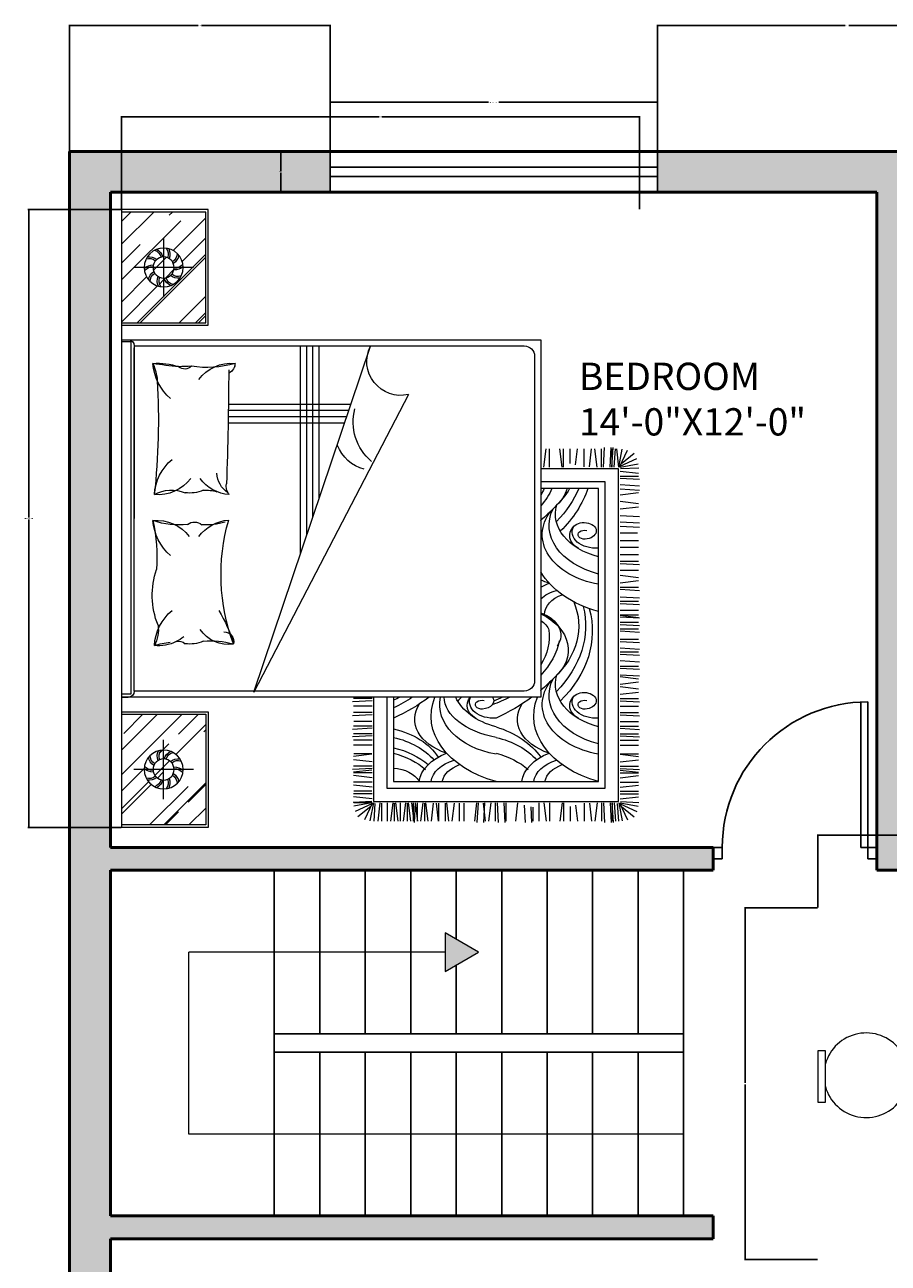
# Model space of a CAD drawing. Units: inches. Extents: x 2831 to 3729, y 3926 to 4974.
# Tile 3 of 8: x 2849 to 3038, y 4702 to 4974. Entities that reach past the tile are written whole.
import ezdxf

# ---------------------------------------------------------------- set-up
doc = ezdxf.new("R2010")
doc.units = ezdxf.units.IN
for name, color, linetype, lineweight in [('A-ANNO-DIMS', 2, 'Continuous', 18), ('A-ANNO-SYMB', 7, 'Continuous', 18), ('A-AREA-IDEN', 7, 'Continuous', 18), ('A-DOOR', 3, 'Continuous', 25), ('A-FLOR-STRS', 7, 'Continuous', 25), ('A-FURN', 8, 'Continuous', 18), ('A-GLAZ', 4, 'Continuous', 25), ('A-WALL', 7, 'Continuous', 50), ('A-WALL-PATT', 252, 'Continuous', 13)]:
    doc.layers.add(name, color=color, linetype=linetype, lineweight=lineweight)
doc.styles.get("Standard").update_dxf_attribs({"font": 'arial.ttf'})
doc.dimstyles.get("Standard").update_dxf_attribs({"dimtxt": 0.18, "dimasz": 0.18, "dimexe": 0.18, "dimexo": 0.0625, "dimgap": 0.09, "dimtad": 0, "dimtih": 1, "dimtoh": 1, "dimdec": 4, "dimzin": 0, "dimdsep": 46, "dimtxsty": 'Standard', "dimcen": 0.09, "dimadec": 0, "dimazin": 0, "dimtfac": 1, "dimtdec": 4, "dimtofl": 0, "dimtmove": 0, "dimatfit": 3, "dimfxl": 1, "dimtolj": 1, "dimtzin": 0, "dimarcsym": 0})

# ---------------------------------------------------------------- blocks, each defined once
blk = doc.blocks.new('A$C709B6AB6')
for p, q in [((0.969, 1.6731), (0.7259, 1.6731)), ((0.7259, 1.6731), (0.7259, 1.6374)), ((0.969, 1.6374), (0.969, 1.6731)), ((1.6452, 1.6731), (1.402, 1.6731)), ((1.402, 1.6731), (1.402, 1.6374)), ((1.6452, 1.6374), (1.6452, 1.6731)), ((0.7259, 1.6374), (0.969, 1.6374)), ((1.402, 1.6374), (1.6452, 1.6374)), ((0.3883, 0.3366), (0.3883, 1.3366)), ((0.3883, 1.3366), (1.9163, 1.3366)), ((0.4919, 1.2463), (0.4015, 1.3366)), ((0.7693, 1.0352), (0.468, 1.3366)), ((0.8475, 1.0774), (0.5883, 1.3366)), ((0.6526, 1.2956), (0.6117, 1.3366)), ((0.8205, 1.1564), (0.6404, 1.3366)), ((1.3746, 0.6706), (0.7087, 1.3366)), ((0.94, 1.1879), (0.7913, 1.3366)), ((1.0576, 1.108), (0.829, 1.3366)), ((1.4563, 0.7595), (0.9175, 1.2983)), ((1.1357, 1.1502), (0.9493, 1.3366)), ((1.2273, 1.0801), (0.9709, 1.3366)), ((1.6629, 0.7434), (1.0697, 1.3366)), ((1.486, 0.9688), (1.1182, 1.3366)), ((1.5147, 0.9724), (1.1505, 1.3366)), ((1.3459, 1.1807), (1.19, 1.3366)), ((1.424, 1.2229), (1.3103, 1.3366)), ((1.8021, 0.8646), (1.3531, 1.3136)), ((1.5156, 1.178), (1.357, 1.3366)), ((1.9163, 0.8509), (1.4307, 1.3366)), ((1.5506, 1.2956), (1.5097, 1.3366)), ((1.6341, 1.2534), (1.551, 1.3366)), ((1.8443, 1.0882), (1.5959, 1.3366)), ((1.7123, 1.2956), (1.6713, 1.3366)), ((1.838, 1.1879), (1.6893, 1.3366)), ((1.9163, 1.2119), (1.7917, 1.3366)), ((1.8739, 1.2974), (1.8348, 1.3366)), ((1.9163, 1.2891), (1.8689, 1.3366)), ((1.9163, 1.3322), (1.912, 1.3366)), ((1.9163, 0.3366), (1.9163, 1.3366)), ((1.0863, 0.5979), (0.3883, 1.296)), ((1.2525, 0.3366), (0.3883, 1.2008)), ((0.7909, 0.9472), (0.5215, 1.2166)), ((1.4321, 0.3366), (0.5448, 1.2238)), ((1.9163, 0.9299), (1.6404, 1.2058)), ((1.9163, 1.0916), (1.8021, 1.2058)), ((0.5592, 1.0047), (0.3883, 1.1756)), ((1.873, 0.7739), (1.5138, 1.1331)), ((1.8146, 0.879), (1.5452, 1.1484)), ((1.9163, 0.9712), (1.7599, 1.1277)), ((0.4622, 1.037), (0.3883, 1.111)), ((1.6117, 0.3366), (0.8322, 1.116)), ((1.4267, 0.5503), (0.8879, 1.0891)), ((0.4811, 0.9625), (0.3883, 1.0553)), ((1.0729, 0.3366), (0.3883, 1.0212)), ((0.7613, 0.738), (0.4919, 1.0074)), ((1.7913, 0.3366), (1.1196, 1.0083)), ((1.5847, 0.7012), (1.2255, 1.0604)), ((1.9163, 0.6102), (1.4716, 1.055)), ((1.9163, 1.0161), (1.9116, 1.0208)), ((0.0357, 0.9927), (0, 0.9927)), ((0, 0.9927), (0, 0.7495)), ((0.0357, 0.7495), (0.0357, 0.9927)), ((1.2965, 0.6284), (0.9373, 0.9876)), ((1.829, 0.3366), (1.1833, 0.9822)), ((2.269, 0.9927), (2.3047, 0.9927)), ((2.269, 0.7495), (2.269, 0.9927)), ((2.3047, 0.9927), (2.3047, 0.7495)), ((0.7981, 0.5251), (0.3883, 0.935)), ((1.0082, 0.5557), (0.649, 0.9149)), ((1.468, 0.3366), (0.8951, 0.9095)), ((1.9163, 0.3911), (1.4069, 0.9005)), ((1.785, 0.6697), (1.5156, 0.9391)), ((0.4326, 0.8278), (0.3883, 0.8721)), ((0.8933, 0.3366), (0.3883, 0.8416)), ((1.107, 0.3366), (0.6068, 0.8368)), ((1.3971, 0.341), (0.8582, 0.8799)), ((0.7199, 0.4829), (0.3883, 0.8146)), ((0.7316, 0.5287), (0.4622, 0.7981)), ((1.9163, 0.5707), (1.6943, 0.7927)), ((1.9163, 0.7773), (1.882, 0.8116)), ((0, 0.7495), (0.0357, 0.7495)), ((1.7554, 0.4605), (1.486, 0.7299)), ((2.3047, 0.7495), (2.269, 0.7495)), ((0.746, 0.3366), (0.3883, 0.6943)), ((0.7136, 0.3366), (0.3883, 0.662)), ((1.1627, 0.3366), (0.8286, 0.6706)), ((1.9163, 0.4899), (1.7527, 0.6536)), ((0.4029, 0.6185), (0.3883, 0.6332)), ((1.9163, 0.5384), (1.8524, 0.6024)), ((0.5098, 0.4524), (0.3883, 0.5739)), ((0.6849, 0.3366), (0.4326, 0.5889)), ((1.7087, 0.3366), (1.4644, 0.5808)), ((1.9163, 0.3696), (1.7105, 0.5754)), ((0.455, 0.4156), (0.3883, 0.4823)), ((1.3477, 0.3366), (1.1761, 0.5081)), ((1.5883, 0.3366), (1.4222, 0.5027)), ((1.6404, 0.3366), (1.4563, 0.5206)), ((0.4317, 0.4102), (0.3883, 0.4536)), ((0.9238, 0.3366), (0.799, 0.4614)), ((0.9866, 0.3366), (0.8879, 0.4353)), ((1.2273, 0.3366), (1.1339, 0.4299)), ((0.446, 0.3366), (0.4029, 0.3797)), ((0.6256, 0.3366), (0.5996, 0.3626)), ((0.8663, 0.3366), (0.8457, 0.3572)), ((1.8793, 0.3366), (1.8227, 0.3931)), ((1.9163, 0.3366), (0.3883, 0.3366)), ((0.7212, 0), (0.7212, 0.0357)), ((0.7212, 0.0357), (0.9644, 0.0357)), ((0.9644, 0.0357), (0.9644, 0)), ((1.3973, 0), (1.3973, 0.0357)), ((1.3973, 0.0357), (1.6405, 0.0357)), ((1.6405, 0.0357), (1.6405, 0)), ((0.9644, 0), (0.7212, 0)), ((1.6405, 0), (1.3973, 0))]:
    blk.add_line(p, q)
for centre, start, end in [((0.8475, 1.4434), 105.52104, 212.06337), ((0.8475, 1.4434), 327.93663, 74.47896), ((1.5236, 1.4434), 105.52104, 212.06337), ((1.5236, 1.4434), 327.93663, 74.47896), ((0.2296, 0.8768), 37.97614, 164.47896), ((2.075, 0.8768), 15.52104, 142.02386), ((0.2296, 0.8768), 195.52104, 322.02386), ((2.075, 0.8768), 217.97614, 344.47896), ((0.8428, 0.2297), 147.93663, 254.47896), ((0.8428, 0.2297), 285.52104, 32.06337), ((1.5189, 0.2297), 147.93663, 254.47896), ((1.5189, 0.2297), 285.52104, 32.06337)]:
    blk.add_arc(centre, 0.2013, start, end)
blk = doc.blocks.new('A$C64B41DC1')
for p, q in [((0, 2.5079), (2.9903, 2.5079)), ((0, 2.0879), (0, 2.5079)), ((0.012, 2.4618), (0.0581, 2.5079)), ((0.012, 2.3515), (0.1684, 2.5079)), ((0.012, 2.0999), (0.012, 2.5079)), ((0.0543, 2.2213), (0.3409, 2.5079)), ((0.1689, 2.4179), (0.2589, 2.5079)), ((0.3265, 2.386), (0.4484, 2.5079)), ((0.3699, 2.3332), (0.5445, 2.5079)), ((0.548, 2.5079), (0.548, 2.0999)), ((0.56, 2.5079), (0.56, 2.0879)), ((0.6301, 2.5079), (0.6301, 0.4779)), ((0.6401, 2.461), (0.6401, 2.5079)), ((0.6401, 2.5079), (2.344, 2.5079)), ((2.344, 2.461), (0.6401, 2.461)), ((2.344, 2.5079), (2.3601, 2.5079)), ((2.344, 2.5079), (2.344, 2.461)), ((2.3601, 2.5079), (2.3601, 2.4761)), ((2.3601, 0.4779), (2.3601, 2.5079)), ((2.4303, 2.5079), (2.4303, 2.0879)), ((2.4423, 2.5079), (2.4423, 2.0999)), ((2.4423, 2.3333), (2.6169, 2.5079)), ((2.4423, 2.2145), (2.7357, 2.5079)), ((2.4423, 2.404), (2.5354, 2.4971)), ((2.705, 2.398), (2.8149, 2.5079)), ((2.7691, 2.3772), (2.8998, 2.5079)), ((2.7819, 2.3646), (2.9252, 2.5079)), ((2.9783, 2.0999), (2.9783, 2.5079)), ((2.9903, 2.0879), (2.9903, 2.5079)), ((0.2157, 2.0999), (0.548, 2.4322)), ((0.2299, 2.0999), (0.548, 2.418)), ((0.2804, 2.1597), (0.2804, 2.4481)), ((0.6601, 2.4461), (1.4951, 2.4461)), ((0.6601, 2.4461), (0.6601, 0.5579)), ((1.4951, 2.4461), (0.6697, 2.4461)), ((2.3301, 2.4461), (1.4951, 2.4461)), ((2.3301, 0.5579), (2.3301, 2.4461)), ((2.7099, 2.1597), (2.7099, 2.4481)), ((0.2311, 2.2906), (0.2937, 2.3532)), ((2.6674, 2.2756), (2.7382, 2.3464)), ((2.7914, 2.1846), (2.9783, 2.3715)), ((0.1362, 2.3039), (0.4246, 2.3039)), ((0.2905, 2.2539), (0.3304, 2.2938)), ((0.3405, 2.3039), (0.3605, 2.3238)), ((2.8541, 2.3039), (2.5657, 2.3039)), ((2.5849, 2.2779), (2.6158, 2.3088)), ((2.6158, 2.3088), (2.6313, 2.3243)), ((2.7249, 2.3076), (2.7512, 2.3339)), ((2.7746, 2.0999), (2.9783, 2.3036)), ((2.9144, 2.2312), (2.9783, 2.2951)), ((0.012, 2.261), (0.0275, 2.2765)), ((0.0404, 2.0999), (0.1982, 2.2578)), ((0.4194, 2.0999), (0.548, 2.2285)), ((2.4423, 2.1353), (2.5382, 2.2312)), ((2.4918, 2.0999), (2.6366, 2.2447)), ((0.1365, 2.0999), (0.251, 2.2144)), ((2.7831, 2.0999), (2.8678, 2.1846)), ((2.8962, 2.0999), (2.9783, 2.182)), ((0.548, 2.0999), (0.012, 2.0999)), ((0.4986, 2.0999), (0.548, 2.1493)), ((0.5127, 2.0999), (0.548, 2.1352)), ((2.4423, 2.0999), (2.9783, 2.0999)), ((2.5172, 2.0999), (2.5269, 2.1096)), ((0.56, 2.0879), (0, 2.0879)), ((2.4303, 2.0879), (2.9903, 2.0879)), ((0.9415, 1.9902), (0.9415, 1.3975)), ((0.9715, 1.9906), (0.9715, 1.4076)), ((1.0015, 1.991), (1.0015, 1.4177)), ((1.0315, 1.9916), (1.0315, 1.4279)), ((2.3349, 1.8678), (0.6613, 1.3029)), ((0.8956, 1.1191), (2.3349, 1.8678)), ((1.6636, 1.6412), (0.6601, 1.6412)), ((1.5748, 1.6112), (0.6601, 1.6112)), ((2.3665, 1.295), (2.3665, 1.3839)), ((2.377, 1.295), (2.3822, 1.3891)), ((2.4032, 1.295), (2.4032, 1.3839)), ((2.4346, 1.295), (2.4346, 1.3839)), ((2.4451, 1.295), (2.4503, 1.3891)), ((2.4774, 1.2957), (2.4774, 1.3837)), ((2.5, 1.295), (2.5, 1.3839)), ((2.5105, 1.295), (2.5157, 1.3891)), ((2.5367, 1.295), (2.5367, 1.3839)), ((2.5471, 1.295), (2.5524, 1.3891)), ((2.5681, 1.295), (2.5681, 1.3839)), ((2.5918, 1.295), (2.5918, 1.3839)), ((2.6346, 1.2957), (2.6346, 1.3837)), ((2.6362, 1.2957), (2.6467, 1.3839)), ((2.6729, 1.295), (2.6624, 1.3839)), ((2.6938, 1.295), (2.6938, 1.3839)), ((2.7043, 1.295), (2.7095, 1.3891)), ((2.7127, 1.2957), (2.7232, 1.3839)), ((2.7253, 1.295), (2.7253, 1.3839)), ((2.7494, 1.295), (2.7389, 1.3839)), ((2.7718, 1.295), (2.7718, 1.3839)), ((2.7959, 1.295), (2.7854, 1.3839)), ((2.8146, 1.2957), (2.8146, 1.3837)), ((2.8146, 1.2957), (2.8146, 1.3837)), ((2.8282, 1.295), (2.8282, 1.3839)), ((2.8282, 1.295), (2.8282, 1.3839)), ((2.8523, 1.295), (2.8418, 1.3839)), ((2.8523, 1.295), (2.8418, 1.3839)), ((2.8653, 1.2966), (2.8688, 1.3861)), ((2.8711, 1.2957), (2.8711, 1.3837)), ((2.8711, 1.2957), (2.8875, 1.3822)), ((2.8713, 1.2927), (2.954, 1.3315)), ((2.8765, 1.2958), (2.9132, 1.3758)), ((2.8893, 1.3011), (2.9394, 1.3636)), ((2.3601, 1.2873), (2.8639, 1.2873)), ((2.8639, 1.2873), (2.8639, 0.1018)), ((2.8716, 1.2565), (2.9605, 1.2669)), ((2.8717, 1.2884), (2.9588, 1.3058)), ((2.8744, 1.2817), (2.9603, 1.2869)), ((2.3601, 1.2233), (2.7999, 1.2233)), ((2.7999, 1.2233), (2.7999, 0.1658)), ((2.8716, 1.2212), (2.9605, 1.2212)), ((2.8716, 1.1947), (2.9605, 1.2052)), ((2.8723, 1.2489), (2.9603, 1.2489)), ((2.3601, 1.1913), (2.7679, 1.1912)), ((2.7679, 1.1912), (2.7679, 0.1978)), ((2.8716, 1.181), (2.9605, 1.1705)), ((2.8716, 1.1595), (2.9605, 1.1595)), ((2.8716, 1.133), (2.9605, 1.1435)), ((2.8723, 1.1872), (2.9603, 1.1872)), ((2.8716, 1.1193), (2.9605, 1.1088)), ((2.8716, 1.1035), (2.9605, 1.093)), ((2.8716, 1.0965), (2.9605, 1.0965)), ((2.8716, 1.086), (2.9657, 1.0913)), ((2.8723, 1.1255), (2.9603, 1.1255)), ((2.8723, 1.0858), (2.9605, 1.0753)), ((2.8716, 1.0756), (2.9605, 1.0756)), ((2.8716, 1.0491), (2.9605, 1.0596)), ((2.8716, 1.0354), (2.9605, 1.0249)), ((2.8723, 1.0416), (2.9603, 1.0416)), ((2.8723, 0.9987), (2.9605, 1.0092)), ((2.8723, 0.985), (2.9605, 0.9745)), ((2.8723, 0.9735), (2.9603, 0.9735)), ((2.8716, 0.9346), (2.9605, 0.9241)), ((2.8723, 0.9408), (2.9603, 0.9408)), ((2.8723, 0.8979), (2.9605, 0.9084)), ((2.8723, 0.8726), (2.9603, 0.8726)), ((2.8723, 0.8505), (2.9603, 0.8505)), ((2.8716, 0.7885), (2.9605, 0.799)), ((2.8716, 0.7818), (2.9657, 0.787)), ((2.8716, 0.7503), (2.9657, 0.7556)), ((2.8716, 0.7204), (2.9605, 0.7309)), ((2.8723, 0.7571), (2.9605, 0.7466)), ((2.8716, 0.6995), (2.9605, 0.6995)), ((2.8716, 0.689), (2.9657, 0.6838)), ((2.8716, 0.6576), (2.9657, 0.6523)), ((2.8716, 0.6471), (2.9605, 0.6471)), ((2.8716, 0.5903), (2.9605, 0.6007)), ((2.882, 0.5582), (2.9657, 0.5536)), ((0.7101, 0.5079), (2.2801, 0.5079)), ((2.8716, 0.4877), (2.9603, 0.4877)), ((2.8909, 0.5263), (2.9657, 0.5222)), ((2.8928, 0.5169), (2.9605, 0.5169)), ((0.6301, 0.4779), (2.3601, 0.4779)), ((1.2465, 0.4625), (1.1576, 0.452)), ((1.2465, 0.4365), (1.1577, 0.4365)), ((1.2542, 0.1018), (1.2542, 0.4779)), ((1.3182, 0.1658), (1.3182, 0.4779)), ((1.3502, 0.1978), (1.3502, 0.4779)), ((2.8716, 0.4625), (2.9605, 0.452)), ((2.8716, 0.4365), (2.9603, 0.4365)), ((1.2465, 0.3746), (1.1576, 0.3851)), ((1.2465, 0.3684), (1.1577, 0.3684)), ((2.8716, 0.3746), (2.9605, 0.3851)), ((2.8716, 0.3684), (2.9603, 0.3684)), ((1.2355, 0.3092), (1.1576, 0.3)), ((1.2285, 0.3357), (1.1577, 0.3357)), ((2.8826, 0.3092), (2.9605, 0.3)), ((2.8896, 0.3357), (2.9603, 0.3357)), ((1.2457, 0.2423), (1.1576, 0.2319)), ((1.2457, 0.2676), (1.1577, 0.2676)), ((2.8723, 0.2676), (2.9603, 0.2676)), ((2.8723, 0.2423), (2.9605, 0.2319)), ((1.2465, 0.2057), (1.1576, 0.2161)), ((1.2465, 0.1847), (1.1576, 0.1847)), ((2.7679, 0.1978), (1.3502, 0.1978)), ((2.8716, 0.2057), (2.9605, 0.2161)), ((2.8716, 0.1847), (2.9605, 0.1847)), ((1.2465, 0.1742), (1.1524, 0.169)), ((1.2465, 0.1428), (1.1524, 0.1376)), ((1.2465, 0.1334), (1.1524, 0.1281)), ((1.2465, 0.1323), (1.1576, 0.1323)), ((1.2465, 0.1323), (1.1576, 0.1323)), ((1.2465, 0.1229), (1.1588, 0.1168)), ((2.7999, 0.1658), (1.3182, 0.1658)), ((2.8716, 0.1742), (2.9657, 0.169)), ((2.8716, 0.1428), (2.9657, 0.1376)), ((2.8716, 0.1334), (2.9657, 0.1281)), ((2.8716, 0.1323), (2.9605, 0.1323)), ((2.8716, 0.1229), (2.9593, 0.1168)), ((1.2465, 0.1), (1.1576, 0.1105)), ((1.2464, 0.1007), (1.1592, 0.0833)), ((1.2468, 0.0964), (1.1641, 0.0576)), ((1.2288, 0.088), (1.1787, 0.0255)), ((1.2415, 0.0933), (1.2049, 0.0133)), ((1.247, 0.0934), (1.2306, 0.0069)), ((1.2527, 0.0925), (1.2493, 0.003)), ((2.8639, 0.1018), (1.2542, 0.1018)), ((1.2658, 0.0941), (1.2762, 0.0052)), ((1.2899, 0.0941), (1.2899, 0.0052)), ((1.2999, 0.0941), (1.3051, 0)), ((1.3313, 0.0941), (1.3365, 0)), ((1.3523, 0.0941), (1.3575, 0)), ((1.3804, 0.0941), (1.3699, 0.0052)), ((1.4119, 0.0934), (1.4223, 0.0052)), ((1.4485, 0.0941), (1.438, 0.0052)), ((1.48, 0.0941), (1.4852, 0)), ((1.5114, 0.0941), (1.5166, 0)), ((1.5323, 0.0941), (1.5376, 0)), ((1.5638, 0.0941), (1.5638, 0.0105)), ((1.6021, 0.0941), (1.6021, 0.0052)), ((1.6336, 0.0941), (1.6336, 0.0052)), ((1.6702, 0.0941), (1.6702, 0.0052)), ((1.7017, 0.0941), (1.7017, 0.0052)), ((1.7122, 0.0941), (1.7174, 0)), ((1.7445, 0.0934), (1.7445, 0.0054)), ((1.7698, 0.0934), (1.7803, 0.0052)), ((1.8065, 0.0941), (1.796, 0.0052)), ((1.8274, 0.0941), (1.8274, 0.0052)), ((1.8379, 0.0941), (1.8431, 0)), ((1.8746, 0.0941), (1.8798, 0)), ((1.8955, 0.0941), (1.8955, 0.0052)), ((1.906, 0.0941), (1.9113, 0)), ((1.9384, 0.0934), (1.9384, 0.0054)), ((1.9609, 0.0941), (1.9609, 0.0052)), ((1.9636, 0.0934), (1.9741, 0.0052)), ((1.9714, 0.0941), (1.9766, 0)), ((1.9976, 0.0941), (1.9976, 0.0052)), ((2.0081, 0.0941), (2.0133, 0)), ((2.029, 0.0941), (2.029, 0.0052)), ((2.0395, 0.0941), (2.0447, 0)), ((2.0797, 0.0941), (2.0797, 0.0052)), ((2.0902, 0.0941), (2.0954, 0)), ((2.1216, 0.0941), (2.1269, 0)), ((2.1412, 0.0941), (2.1412, 0.0052)), ((2.1517, 0.0941), (2.1569, 0)), ((2.1831, 0.0941), (2.1884, 0)), ((2.2093, 0.0941), (2.2093, 0.0052)), ((2.2198, 0.0941), (2.225, 0)), ((2.2512, 0.0941), (2.2565, 0)), ((2.2603, 0.0934), (2.2707, 0.0052)), ((2.2969, 0.0941), (2.2864, 0.0052)), ((2.3089, 0.0934), (2.3193, 0.0052)), ((2.3455, 0.0941), (2.3351, 0.0052)), ((2.3665, 0.0941), (2.3665, 0.0052)), ((2.377, 0.0941), (2.3822, 0)), ((2.4032, 0.0941), (2.4032, 0.0052)), ((2.4346, 0.0941), (2.4346, 0.0052)), ((2.4451, 0.0941), (2.4503, 0)), ((2.4774, 0.0934), (2.4774, 0.0054)), ((2.5, 0.0941), (2.5, 0.0052)), ((2.5105, 0.0941), (2.5157, 0)), ((2.5367, 0.0941), (2.5367, 0.0052)), ((2.5471, 0.0941), (2.5524, 0)), ((2.5681, 0.0941), (2.5681, 0.0052)), ((2.5918, 0.0941), (2.5918, 0.0052)), ((2.6346, 0.0934), (2.6346, 0.0054)), ((2.6362, 0.0934), (2.6467, 0.0052)), ((2.6729, 0.0941), (2.6624, 0.0052)), ((2.6938, 0.0941), (2.6938, 0.0052)), ((2.7043, 0.0941), (2.7095, 0)), ((2.7127, 0.0934), (2.7232, 0.0052)), ((2.7253, 0.0941), (2.7253, 0.0052)), ((2.7494, 0.0941), (2.7389, 0.0052)), ((2.7718, 0.0941), (2.7718, 0.0052)), ((2.7959, 0.0941), (2.7854, 0.0052)), ((2.8146, 0.0934), (2.8146, 0.0054)), ((2.8282, 0.0941), (2.8282, 0.0052)), ((2.8523, 0.0941), (2.8418, 0.0052)), ((2.8653, 0.0925), (2.8688, 0.003)), ((2.8711, 0.0934), (2.8875, 0.0069)), ((2.8713, 0.0964), (2.954, 0.0576)), ((2.8717, 0.1007), (2.9588, 0.0833)), ((2.8744, 0.1074), (2.9603, 0.1022)), ((2.8765, 0.0933), (2.9132, 0.0133)), ((2.8893, 0.088), (2.9394, 0.0255))]:
    blk.add_line(p, q)
at = {"ltscale": 10}
for p, q in [((1.4859, 1.5812), (0.6601, 1.5812)), ((1.397, 1.5512), (0.6601, 1.5512))]:
    blk.add_line(p, q, dxfattribs=at)
for centre, radius in [((0.2804, 2.3039), 0.0942), ((2.7099, 2.3039), 0.0942), ((0.2804, 2.3039), 0.051), ((2.7099, 2.3039), 0.051)]:
    blk.add_circle(centre, radius)
for centre, radius, start, end in [((0.6601, 2.4761), 0.03, 180, 270), ((2.3301, 2.4761), 0.03, 270, 0), ((0.3286, 2.3561), 0.0605, 136.17003, 182.48975), ((2.6617, 2.3561), 0.0605, 357.51025, 43.82997), ((0.2417, 2.3614), 0.0462, 196.30017, 256.53802), ((0.2887, 2.3745), 0.0605, 172.17003, 218.48975), ((0.2828, 2.3731), 0.0462, 160.30017, 220.53802), ((0.3231, 2.3585), 0.0462, 124.30017, 184.53802), ((0.3501, 2.3178), 0.0605, 100.17003, 146.48975), ((0.347, 2.323), 0.0462, 88.30017, 148.53802), ((1.0526, 2.3302), 0.3085, 175.30484, 198.69419), ((-0.8702, 2.0941), 1.6364, 4.80985, 9.18918), ((0.8579, 2.6278), 0.2948, 247.51785, 264.26696), ((0.728, 2.111), 0.245, 40.4189, 85.9871), ((1.0164, 5.7096), 3.3803, 266.81337, 276.16021), ((1.3963, 2.1044), 0.245, 94.0129, 139.5811), ((1.1858, 2.3288), 0.1943, 306.5711, 5.88998), ((1.5348, 2.2652), 0.1767, 151.77364, 201.69827), ((1.6986, 2.3355), 0.1943, 174.11002, 233.4289), ((1.1481, 2.2311), 0.3783, 353.49469, 19.18669), ((1.6871, 3.192), 0.8561, 257.74383, 273.62843), ((1.4882, 2.111), 0.245, 40.4189, 85.9871), ((1.8674, 1.9709), 0.3878, 68.20259, 108.9817), ((2.1269, 2.1044), 0.245, 94.0129, 139.5811), ((2.0342, 2.4856), 0.1563, 261.59582, 298.90918), ((1.9165, 2.3288), 0.1943, 333.73715, 5.88998), ((2.6058, 2.2028), 0.517, 163.60457, 172.3273), ((2.6433, 2.323), 0.0462, 31.46198, 91.69983), ((2.6402, 2.3178), 0.0605, 33.51025, 79.82997), ((2.6672, 2.3585), 0.0462, 355.46198, 55.69983), ((2.7075, 2.3731), 0.0462, 319.46198, 19.69983), ((2.7016, 2.3745), 0.0605, 321.51025, 7.82997), ((2.7486, 2.3614), 0.0462, 283.46198, 343.69983), ((0.2153, 2.3276), 0.0462, 232.30017, 292.53802), ((0.2158, 2.3336), 0.0605, 244.17003, 290.48975), ((0.2457, 2.3659), 0.0605, 208.17003, 254.48975), ((0.3449, 2.2742), 0.0605, 64.17003, 110.48975), ((0.3455, 2.2802), 0.0462, 52.30017, 112.53802), ((0.3191, 2.2464), 0.0462, 16.30017, 76.53802), ((0.3151, 2.2419), 0.0605, 28.17003, 74.48975), ((2.6448, 2.2802), 0.0462, 67.46198, 127.69983), ((2.6454, 2.2742), 0.0605, 69.51025, 115.82997), ((2.6752, 2.2419), 0.0605, 105.51025, 151.82997), ((2.6712, 2.2464), 0.0462, 103.46198, 163.69983), ((2.7744, 2.3336), 0.0605, 249.51025, 295.82997), ((2.775, 2.3276), 0.0462, 247.46198, 307.69983), ((2.7446, 2.3659), 0.0605, 285.51025, 331.82997), ((0.2138, 2.2848), 0.0462, 268.30017, 328.53802), ((0.2107, 2.29), 0.0605, 280.17003, 326.48975), ((0.2377, 2.2493), 0.0462, 304.30017, 4.53802), ((0.2322, 2.2517), 0.0605, 316.17003, 2.48975), ((0.2779, 2.2347), 0.0462, 340.30017, 40.53802), ((0.272, 2.2333), 0.0605, 352.17003, 38.48975), ((0.7274, 2.2013), 0.0446, 314.4736, 42.17134), ((-1.6008, 2.277), 2.3618, 357.39054, 358.88764), ((1.9165, 2.3288), 0.1943, 320.94042, 333.73715), ((2.1347, 2.2313), 0.0459, 165.35061, 223.26844), ((2.7182, 2.2333), 0.0605, 141.51025, 187.82997), ((2.7123, 2.2347), 0.0462, 139.46198, 199.69983), ((2.7581, 2.2517), 0.0605, 177.51025, 223.82997), ((2.7526, 2.2493), 0.0462, 175.46198, 235.69983), ((2.7796, 2.29), 0.0605, 213.51025, 259.82997), ((2.7765, 2.2848), 0.0462, 211.46198, 271.69983), ((0.2688, 2.0945), 0.4956, 344.0243, 8.70709), ((1.204, 2.1778), 0.1681, 337.01697, 7.53676), ((1.5671, 2.1546), 0.0547, 142.08329, 220.902), ((1.9346, 2.1778), 0.1681, 337.01697, 7.53676), ((0.9385, 1.978), 0.1943, 126.5711, 185.88998), ((1.1858, 1.9714), 0.1943, 4.31813, 53.4289), ((1.5415, 2.0969), 0.1834, 175.22328, 196.23004), ((1.7059, 1.9714), 0.204, 127.11975, 175.09005), ((1.1965, 2.0983), 0.3299, 343.79543, 3.55541), ((1.9394, 1.991), 0.1651, 351.26213, 55.75721), ((2.4617, 2.0719), 0.3745, 173.82958, 196.4356), ((1.2687, 1.9248), 0.1223, 33.62799, 86.47438), ((0.7417, 2.0149), 0.057, 273.47085, 328.54118), ((0.7246, 18.8439), 16.8552, 270.17399, 272.05214), ((1.3401, 1.9404), 0.0603, 49.09906, 101.37023), ((1.7676, 1.0629), 0.9631, 69.65065, 105.96307), ((2.2748, 2.5795), 0.6373, 238.34989, 254.31375), ((2.0911, 2.0123), 0.0478, 179.77267, 283.80184), ((0.728, 2.2025), 0.245, 274.0129, 278.34166), ((1.0747, 1.2871), 0.1871, 14.1863, 69.12121), ((1.0274, 1.1334), 0.2527, 40.62904, 104.37123), ((0.7347, 1.1553), 0.1649, 347.31088, 116.44537), ((0.7101, 0.5579), 0.05, 180, 270), ((2.2801, 0.5579), 0.05, 270, 0)]:
    blk.add_arc(centre, radius, start, end)
for centre, major_axis, ratio, start_param, end_param in [((1.9938, 1.6262), (0, -0.7531), 0.68, 0.797284, 0.954936), ((2.0643, 1.466), (0, -0.5322), 0.68, 7.239912, 7.311536), ((1.9052, 1.7397), (0, -0.9842), 0.68, 0.74745, 0.979724), ((2.7455, 1.3081), (0, 0.3614), 0.68, 1.900046, 2.742661), ((2.7868, 1.3081), (0, 0.3614), 0.68, 1.900046, 2.614747), ((2.8372, 1.3081), (0, 0.3614), 0.68, 1.900046, 2.479658), ((2.8607, 1.3211), (0, 0.3614), 0.68, 1.938265, 2.479658), ((2.8057, 1.2079), (0, -0.1524), 0.68, 4.821745, 5.895886), ((2.4665, 0.8216), (0, -0.2664), 0.68, 2.006169, 3.565187), ((2.4513, 0.5069), (0, 0.502), 0.68, 5.095327, 6.553458), ((2.7862, 0.8069), (0, -0.2615), 0.68, 3.244645, 4.205018), ((2.396, 0.6032), (0, 0.3641), 0.68, -1.3172, 0.145284), ((2.7784, 0.8289), (0, -0.1802), 0.68, 3.227058, 4.318474), ((2.3507, 0.5642), (0.0073, 0.3819), 0.56205, -1.21172, -0.009991), ((2.7821, 0.7971), (0, -0.1589), 0.68, 3.272942, 4.229533), ((2.2964, 0.5771), (0, -0.3263), 0.68, 1.938944, 2.850232), ((2.0403, 1.6015), (0, -0.8763), 0.68, 6.849801, 6.887077), ((2.4005, 0.7132), (0, -0.1214), 0.68, 2.284368, 3.652258), ((2.3834, 0.7081), (0, 0.1147), 0.68, 4.593909, 6.585576), ((2.3961, 0.7628), (0, -0.0317), 0.68, 1.462497, 5.046281), ((2.3774, 0.7653), (0, -0.0593), 0.68, 5.841311, 7.755362), ((1.9938, 1.1295), (-0.0678, 0.7439), 0.610498, 3.917146, 4.063997), ((2.0643, 0.9693), (0, -0.5322), 0.68, 7.239912, 7.336618), ((1.9052, 1.243), (0, -0.9842), 0.68, 0.74745, 0.979724), ((2.7455, 0.8114), (-0.0599, 0.3735), 0.695517, 1.775813, 2.548612), ((2.7868, 0.8114), (0, 0.3614), 0.68, 1.900046, 2.614747), ((2.8607, 0.8243), (0, 0.3614), 0.68, 1.938265, 2.479658), ((2.4665, 0.3249), (0, -0.2664), 0.68, 2.006169, 3.565187), ((2.4513, 0.0102), (0, 0.502), 0.68, 5.095327, 6.553458), ((2.7862, 0.3102), (0, -0.2615), 0.68, 3.244645, 4.205018), ((1.5283, 0.0674), (0, -0.3703), 0.68, 1.930561, 3.464283), ((1.5736, 0.1065), (0, 0.3641), 0.68, -1.3172, 0.476403), ((2.3507, 0.0674), (0, -0.3703), 0.68, 1.930561, 3.464283), ((2.396, 0.1065), (0, 0.3641), 0.68, -1.3172, 0.476403), ((2.7784, 0.3322), (0, -0.1802), 0.68, 3.227058, 4.318474), ((1.242, 0.9693), (0, -0.5322), 0.68, 6.586764, 6.677612), ((1.1714, 1.1295), (-0.1157, 0.7241), 0.59432, 3.291697, 3.50733), ((1.474, 0.0804), (0, -0.3263), 0.68, 1.938944, 3.339184), ((1.0828, 1.243), (0, -0.9842), 0.68, 0.565948, 0.680366), ((1.6289, 0.0102), (0, 0.502), 0.68, 6.655152, 6.661293), ((1.6289, 0.0102), (0, 0.502), 0.68, 5.095327, 5.911219), ((1.6442, 0.3249), (0, -0.2664), 0.68, 2.006169, 2.182797), ((1.9638, 0.3102), (0, -0.2615), 0.68, 4.015924, 4.205018), ((1.956, 0.3322), (0, -0.1802), 0.68, 3.770744, 4.318474), ((1.9597, 0.3004), (0, -0.1589), 0.68, 3.14258, 4.229533), ((2.0606, 0.5616), (0, -0.1803), 0.68, 5.194792, 5.929328), ((2.0606, 0.5616), (0, -0.1803), 0.68, 5.194792, 6.723255), ((2.1315, 0.6603), (0, -0.3155), 0.68, 5.328638, 6.949396), ((2.0549, 0.5656), (0, -0.1303), 0.68, 5.450951, 6.054641), ((2.0643, 0.9693), (0, -0.5322), 0.68, 6.20013, 6.677612), ((1.9938, 1.1295), (-0.0678, 0.7439), 0.610498, 3.199135, 3.592282), ((2.2964, 0.0804), (0, -0.3263), 0.68, 1.938944, 3.339184), ((1.9052, 1.243), (0, -0.9842), 0.68, 0.565948, 0.680366), ((2.4513, 0.0102), (0, 0.502), 0.68, 6.655152, 6.661293), ((2.7821, 0.3004), (0, -0.1589), 0.68, 3.272942, 4.229533), ((1.1933, 0.9181), (0, -0.624), 0.68, 0.378672, 0.625379), ((1.3091, 0.6603), (0, -0.3155), 0.68, 6.475719, 6.949396), ((1.1911, 1.1066), (0, 0.8458), 0.68, 3.421828, 3.728616), ((1.2179, 1.1047), (0, -0.8763), 0.68, 6.507006, 6.887077), ((2.0157, 0.9181), (0, -0.624), 0.68, -0.280078, 0.625379), ((2.0135, 1.1066), (0, 0.8458), 0.68, 2.978727, 3.728616), ((2.0403, 1.1047), (0, -0.8763), 0.68, 6.099302, 6.887077), ((1.555, 0.2685), (0, -0.0593), 0.68, 3.732151, 7.755362), ((1.5781, 0.2165), (0, -0.1214), 0.68, 2.284368, 3.726131), ((1.561, 0.2114), (0, 0.1147), 0.68, 4.593909, 6.647252), ((1.5737, 0.2661), (0, -0.0317), 0.68, 1.462497, 5.046281), ((2.3774, 0.2685), (0, -0.0593), 0.68, 3.732151, 7.755362), ((2.4005, 0.2165), (0, -0.1214), 0.68, 2.284368, 3.726131), ((2.3834, 0.2114), (0, 0.1147), 0.68, 4.593909, 6.647252), ((2.3961, 0.2661), (0, -0.0317), 0.68, 1.462497, 5.046281)]:
    blk.add_ellipse(centre, major_axis=major_axis, ratio=ratio, start_param=start_param, end_param=end_param)
blk = doc.blocks.new('DOOR-SWING-32IN')
for p, q in [((-32, 2.5), (-34, 2.5)), ((-34, 0), (-32, 0)), ((-32, 0), (-32, 2.5)), ((0, 0), (0, 2.5)), ((0, 2.5), (2, 2.5)), ((2, 0), (0, 0)), ((-1.5, 0), (-1.5, -31.96)), ((0, 0), (-1.5, 0)), ((0, 0), (0, -32))]:
    blk.add_line(p, q)
blk.add_arc((0, 0), 32, 180, 270)
blk = doc.blocks.new('WINDOW-72IN-PLAN')
for p, q in [((0, 0), (0, 9)), ((72, 0), (72, 9)), ((72, 5.5), (0, 5.5)), ((72, 3.5), (0, 3.5))]:
    blk.add_line(p, q)
blk = doc.blocks.new('STAIR-HALF-TURN')
for p, q in [((0, 76), (0, 40)), ((10, 76), (10, 40)), ((20, 76), (20, 40)), ((30, 76), (30, 40)), ((40, 76), (40, 60.82)), ((50, 76), (50, 40)), ((60, 76), (60, 40)), ((70, 76), (70, 40)), ((80, 76), (80, 40)), ((90, 76), (90, 40)), ((40, 55.18), (40, 40)), ((90, 40), (0, 40)), ((0, 36), (0, 40)), ((90, 36), (90, 40)), ((90, 36), (0, 36)), ((0, 36), (0, 0)), ((10, 36), (10, 0)), ((20, 36), (20, 0)), ((30, 36), (30, 0)), ((40, 36), (40, 0)), ((50, 36), (50, 0)), ((60, 36), (60, 0)), ((70, 36), (70, 0)), ((80, 36), (80, 0)), ((90, 36), (90, 0))]:
    blk.add_line(p, q)
blk = doc.blocks.new('STAIR-DIRECTION')
h = blk.add_hatch(color=256)
h.dxf.hatch_style = 1
h.paths.add_polyline_path([(63.65, 40), (56.32, 44.24), (56.32, 35.76)])
for p, q in [((0, 0), (0, 40)), ((56.32, 40), (0, 40)), ((108.76, 0), (0, 0))]:
    blk.add_line(p, q)
blk.add_lwpolyline([(63.65, 40), (56.32, 44.24), (56.32, 35.76)], close=True)
blk = doc.blocks.new('*D23')
at = {"layer": 'A-ANNO-DIMS', "color": 0, "lineweight": -2, "transparency": 16777216}
for p, q in [((2915.74, 4946.2), (2915.74, 4957.12)), ((2915.92, 4956.94), (2950.62, 4956.94)), ((2987.56, 4956.94), (2952.86, 4956.94)), ((2987.74, 4946.2), (2987.74, 4957.12))]:
    blk.add_line(p, q, dxfattribs=at)
at = {"layer": 'A-ANNO-DIMS', "color": 0, "transparency": 16777216}
for points in [[(2915.92, 4956.97), (2915.92, 4956.91), (2915.74, 4956.94)], [(2987.56, 4956.97), (2987.56, 4956.91), (2987.74, 4956.94)]]:
    blk.add_solid(points, dxfattribs=at)
at = {"layer": 'Defpoints', "color": 0, "transparency": 16777216}
for p in [(2987.74, 4956.94), (2915.74, 4946.14), (2987.74, 4946.14)]:
    blk.add_point(p, dxfattribs=at)
at = {"layer": 'A-ANNO-DIMS', "color": 0, "transparency": 16777216, "insert": (2951.74, 4956.94), "char_height": 0.18, "attachment_point": 5}
blk.add_mtext('\\A1;WINDOW 72 TYP.', dxfattribs=at)
blk = doc.blocks.new('*D24')
at = {"layer": 'A-ANNO-DIMS', "color": 0, "lineweight": -2, "transparency": 16777216}
for p, q in [((2915.68, 4946.14), (2904.76, 4946.14)), ((2904.94, 4945.96), (2904.94, 4941.82)), ((2904.94, 4937.32), (2904.94, 4941.46)), ((2915.68, 4937.14), (2904.76, 4937.14))]:
    blk.add_line(p, q, dxfattribs=at)
at = {"layer": 'A-ANNO-DIMS', "color": 0, "transparency": 16777216}
for points in [[(2904.91, 4945.96), (2904.97, 4945.96), (2904.94, 4946.14)], [(2904.91, 4937.32), (2904.97, 4937.32), (2904.94, 4937.14)]]:
    blk.add_solid(points, dxfattribs=at)
at = {"layer": 'Defpoints', "color": 0, "transparency": 16777216}
for p in [(2904.94, 4946.14), (2915.74, 4946.14), (2915.74, 4937.14)]:
    blk.add_point(p, dxfattribs=at)
at = {"layer": 'A-ANNO-DIMS', "color": 0, "transparency": 16777216, "insert": (2904.94, 4941.64), "char_height": 0.18, "attachment_point": 5}
blk.add_mtext('\\A1;9 TYP.', dxfattribs=at)
blk = doc.blocks.new('*D35')
at = {"layer": 'A-ANNO-DIMS', "color": 0, "lineweight": -2, "transparency": 16777216}
for p, q in [((2869.82, 4933.36), (2849.33, 4933.36)), ((2849.51, 4933.18), (2849.51, 4865.63)), ((2849.51, 4797.72), (2849.51, 4865.26)), ((2869.82, 4797.54), (2849.33, 4797.54))]:
    blk.add_line(p, q, dxfattribs=at)
at = {"layer": 'A-ANNO-DIMS', "color": 0, "transparency": 16777216}
for points in [[(2849.48, 4933.18), (2849.54, 4933.18), (2849.51, 4933.36)], [(2849.48, 4797.72), (2849.54, 4797.72), (2849.51, 4797.54)]]:
    blk.add_solid(points, dxfattribs=at)
at = {"layer": 'Defpoints', "color": 0, "transparency": 16777216}
for p in [(2869.88, 4933.36), (2849.51, 4797.54), (2869.88, 4797.54)]:
    blk.add_point(p, dxfattribs=at)
at = {"layer": 'A-ANNO-DIMS', "color": 0, "transparency": 16777216, "insert": (2849.51, 4865.45), "char_height": 0.18, "attachment_point": 5}
blk.add_mtext('\\A1;BED GROUP 136', dxfattribs=at)
blk = doc.blocks.new('*D36')
at = {"layer": 'A-ANNO-DIMS', "color": 0, "lineweight": -2, "transparency": 16777216}
for p, q in [((2869.88, 4933.42), (2869.88, 4953.91)), ((2870.06, 4953.73), (2926.56, 4953.73)), ((2983.62, 4953.73), (2927.12, 4953.73)), ((2983.8, 4933.42), (2983.8, 4953.91))]:
    blk.add_line(p, q, dxfattribs=at)
at = {"layer": 'A-ANNO-DIMS', "color": 0, "transparency": 16777216}
for points in [[(2870.06, 4953.76), (2870.06, 4953.7), (2869.88, 4953.73)], [(2983.62, 4953.76), (2983.62, 4953.7), (2983.8, 4953.73)]]:
    blk.add_solid(points, dxfattribs=at)
at = {"layer": 'Defpoints', "color": 0, "transparency": 16777216}
for p in [(2869.88, 4953.73), (2869.88, 4933.36), (2983.8, 4933.36)]:
    blk.add_point(p, dxfattribs=at)
at = {"layer": 'A-ANNO-DIMS', "color": 0, "transparency": 16777216, "insert": (2926.84, 4953.73), "char_height": 0.18, "attachment_point": 5}
blk.add_mtext('\\A1;114', dxfattribs=at)
blk = doc.blocks.new('*D41')
at = {"layer": 'A-ANNO-DIMS', "color": 0, "lineweight": -2, "transparency": 16777216}
for p, q in [((3023.02, 4779.92), (3023.02, 4796.01)), ((3023.2, 4795.83), (3075.24, 4795.83)), ((3129.35, 4795.83), (3077.31, 4795.83)), ((3129.53, 4779.92), (3129.53, 4796.01))]:
    blk.add_line(p, q, dxfattribs=at)
at = {"layer": 'A-ANNO-DIMS', "color": 0, "transparency": 16777216}
for points in [[(3023.2, 4795.86), (3023.2, 4795.8), (3023.02, 4795.83)], [(3129.35, 4795.86), (3129.35, 4795.8), (3129.53, 4795.83)]]:
    blk.add_solid(points, dxfattribs=at)
at = {"layer": 'Defpoints', "color": 0, "transparency": 16777216}
for p in [(3129.53, 4795.83), (3023.02, 4779.86), (3129.53, 4779.86)]:
    blk.add_point(p, dxfattribs=at)
at = {"layer": 'A-ANNO-DIMS', "color": 0, "transparency": 16777216, "insert": (3076.27, 4795.83), "char_height": 0.18, "attachment_point": 5}
blk.add_mtext('\\A1;DINING SET 107', dxfattribs=at)
blk = doc.blocks.new('*D42')
at = {"layer": 'A-ANNO-DIMS', "color": 0, "lineweight": -2, "transparency": 16777216}
for p, q in [((3022.96, 4779.86), (3006.87, 4779.86)), ((3007.05, 4779.68), (3007.05, 4741.38)), ((3007.05, 4702.72), (3007.05, 4741.02)), ((3022.96, 4702.54), (3006.87, 4702.54))]:
    blk.add_line(p, q, dxfattribs=at)
at = {"layer": 'A-ANNO-DIMS', "color": 0, "transparency": 16777216}
for points in [[(3007.02, 4779.68), (3007.08, 4779.68), (3007.05, 4779.86)], [(3007.02, 4702.72), (3007.08, 4702.72), (3007.05, 4702.54)]]:
    blk.add_solid(points, dxfattribs=at)
at = {"layer": 'Defpoints', "color": 0, "transparency": 16777216}
for p in [(3007.05, 4779.86), (3023.02, 4779.86), (3023.02, 4702.54)]:
    blk.add_point(p, dxfattribs=at)
at = {"layer": 'A-ANNO-DIMS', "color": 0, "transparency": 16777216, "insert": (3007.05, 4741.2), "char_height": 0.18, "attachment_point": 5}
blk.add_mtext('\\A1;77', dxfattribs=at)
blk = doc.blocks.new('*D51')
at = {"layer": 'A-ANNO-DIMS', "color": 0, "lineweight": -2, "transparency": 16777216}
for p, q in [((2858.49, 4946.2), (2858.49, 4973.97)), ((2858.67, 4973.79), (2886.72, 4973.79)), ((2915.56, 4973.79), (2887.51, 4973.79)), ((2915.74, 4946.2), (2915.74, 4973.97))]:
    blk.add_line(p, q, dxfattribs=at)
at = {"layer": 'A-ANNO-DIMS', "color": 0, "transparency": 16777216}
for points in [[(2858.67, 4973.82), (2858.67, 4973.76), (2858.49, 4973.79)], [(2915.56, 4973.82), (2915.56, 4973.76), (2915.74, 4973.79)]]:
    blk.add_solid(points, dxfattribs=at)
at = {"layer": 'Defpoints', "color": 0, "transparency": 16777216}
for p in [(2915.74, 4973.79), (2858.49, 4946.14), (2915.74, 4946.14)]:
    blk.add_point(p, dxfattribs=at)
at = {"layer": 'A-ANNO-DIMS', "color": 0, "transparency": 16777216, "insert": (2887.12, 4973.79), "char_height": 0.18, "attachment_point": 5}
blk.add_mtext('\\A1;57.25', dxfattribs=at)
blk = doc.blocks.new('*D52')
at = {"layer": 'A-ANNO-DIMS', "color": 0, "lineweight": -2, "transparency": 16777216}
for p, q in [((2987.74, 4946.2), (2987.74, 4973.97)), ((2987.92, 4973.79), (3029.03, 4973.79)), ((3070.94, 4973.79), (3029.82, 4973.79)), ((3071.12, 4946.2), (3071.12, 4973.97))]:
    blk.add_line(p, q, dxfattribs=at)
at = {"layer": 'A-ANNO-DIMS', "color": 0, "transparency": 16777216}
for points in [[(2987.92, 4973.82), (2987.92, 4973.76), (2987.74, 4973.79)], [(3070.94, 4973.82), (3070.94, 4973.76), (3071.12, 4973.79)]]:
    blk.add_solid(points, dxfattribs=at)
at = {"layer": 'Defpoints', "color": 0, "transparency": 16777216}
for p in [(3071.12, 4973.79), (2987.74, 4946.14), (3071.12, 4946.14)]:
    blk.add_point(p, dxfattribs=at)
at = {"layer": 'A-ANNO-DIMS', "color": 0, "transparency": 16777216, "insert": (3029.43, 4973.79), "char_height": 0.18, "attachment_point": 5}
blk.add_mtext('\\A1;83.38', dxfattribs=at)

msp = doc.modelspace()

# ---------------------------------------------------------------- hatches: boundary and pattern name
at = {"layer": 'A-WALL-PATT'}
h = msp.add_hatch(color=256, dxfattribs=at)
h.dxf.hatch_style = 1
h.paths.add_polyline_path([(2867.4912, 4707.1405), (2999.9912, 4707.1405), (2999.9912, 4712.1405), (2867.4912, 4712.1405), (2867.4912, 4788.1405), (2999.9912, 4788.1405), (2999.9912, 4793.1405), (2867.4912, 4793.1405), (2867.4912, 4937.1405), (2915.7412, 4937.1405), (2915.7412, 4946.1405), (2858.4912, 4946.1405), (2858.4912, 4526.1405), (2895.7412, 4526.1405), (2895.7412, 4535.1405), (2867.4912, 4535.1405)])
h.paths.add_polyline_path([(3071.1162, 4946.1405), (2987.7412, 4946.1405), (2987.7412, 4937.1405), (3035.9912, 4937.1405), (3035.9912, 4788.1405), (3101.2412, 4788.1405), (3101.2412, 4793.1405), (3040.9912, 4793.1405), (3040.9912, 4937.1405), (3071.1162, 4937.1405)])

# ---------------------------------------------------------------- linework, layer by layer
at = {"layer": 'A-WALL'}
for p, q in [((2858.4912, 4946.1405), (3218.4912, 4946.1405)), ((2858.4912, 4946.1405), (2858.4912, 4466.1405)), ((2867.4912, 4937.1405), (3035.9912, 4937.1405)), ((2867.4912, 4937.1405), (2867.4912, 4793.1405)), ((3035.9912, 4937.1405), (3035.9912, 4788.1405)), ((2867.4912, 4793.1405), (2999.9912, 4793.1405)), ((2999.9912, 4793.1405), (2999.9912, 4788.1405)), ((2867.4912, 4788.1405), (2999.9912, 4788.1405)), ((2867.4912, 4788.1405), (2867.4912, 4712.1405)), ((3035.9912, 4788.1405), (3101.2412, 4788.1405)), ((2867.4912, 4712.1405), (2999.9912, 4712.1405)), ((2999.9912, 4712.1405), (2999.9912, 4707.1405)), ((2867.4912, 4707.1405), (2999.9912, 4707.1405)), ((2867.4912, 4707.1405), (2867.4912, 4535.1405))]:
    msp.add_line(p, q, dxfattribs=at)

# ---------------------------------------------------------------- block references
at = {"layer": 'A-ANNO-SYMB'}
msp.add_blockref('STAIR-DIRECTION', (2884.729, 4730.1405), dxfattribs=at)
at = {"layer": 'A-DOOR', "extrusion": (0, 0, -1), "zscale": -1, "rotation": 180}
msp.add_blockref('DOOR-SWING-32IN', (-3033.9912, 4793.1405), dxfattribs=at)
at = {"layer": 'A-FLOR-STRS'}
msp.add_blockref('STAIR-HALF-TURN', (2903.4912, 4712.1405), dxfattribs=at)
at = {"layer": 'A-FURN', "xscale": -45.42195783316389, "yscale": 45.42195783316389, "zscale": 45.42195783316389, "rotation": 90}
msp.add_blockref('A$C64B41DC1', (2983.7978, 4933.3597), dxfattribs=at)
at = {"layer": 'A-FURN', "xscale": 46.21065113701777, "yscale": 46.21065113701777, "zscale": 46.21065113701777}
msp.add_blockref('A$C709B6AB6', (3023.0222, 4702.5423), dxfattribs=at)
at = {"layer": 'A-GLAZ'}
msp.add_blockref('WINDOW-72IN-PLAN', (2915.7412, 4937.1405), dxfattribs=at)

# ---------------------------------------------------------------- texts
at = {"layer": 'A-AREA-IDEN', "insert": (2970.4784, 4899.6911), "char_height": 6, "attachment_point": 1}
msp.add_mtext_dynamic_manual_height_columns('BEDROOM \\P14\'-0"X12\'-0"', width=75.661105, gutter_width=12.5, heights=[0], dxfattribs=at)

# ---------------------------------------------------------------- dimensions: what is measured, and where the dimension line sits
at = {"layer": 'A-ANNO-DIMS'}
for base, p1, p2, picture, middle in [((2915.7412, 4973.7905), (2858.4912, 4946.1405), (2915.7412, 4946.1405), '*D51', (2887.1162, 4973.7905)), ((3071.116169, 4973.790495), (2987.741169, 4946.140495), (3071.116169, 4946.140495), '*D52', (3029.428669, 4973.790495))]:
    dim = msp.add_linear_dim(base=base, p1=p1, p2=p2, dimstyle='Standard', override={"dimdec": 2, "dimlfac": 1, "dimrnd": 0, "dimzin": 0, "dimdsep": 46, "dimlunit": 2}, dxfattribs=at)
    dim.commit()
    dim.dimension.update_dxf_attribs({"geometry": picture, "text_midpoint": middle})
for base, p1, p2, text, picture, middle in [((2987.7412, 4956.9405), (2915.7412, 4946.1405), (2987.7412, 4946.1405), 'WINDOW <> TYP.', '*D23', (2951.7412, 4956.9405)), ((3129.5255, 4795.8345), (3023.0222, 4779.8591), (3129.5255, 4779.8591), 'DINING SET <>', '*D41', (3076.2739, 4795.8345))]:
    dim = msp.add_linear_dim(base=base, p1=p1, p2=p2, text=text, dimstyle='Standard', override={"dimdec": 0, "dimlfac": 1, "dimrnd": 0, "dimzin": 0, "dimdsep": 46, "dimlunit": 2}, dxfattribs=at)
    dim.commit()
    dim.dimension.update_dxf_attribs({"geometry": picture, "text_midpoint": middle})
for base, p1, p2, angle, picture, middle in [((2869.8839, 4953.7334), (2983.7978, 4933.3597), (2869.8839, 4933.3597), 180, '*D36', (2926.8408, 4953.7334)), ((3007.0467, 4779.8591), (3023.0222, 4702.5423), (3023.0222, 4779.8591), 90, '*D42', (3007.0467, 4741.2007))]:
    dim = msp.add_linear_dim(base=base, p1=p1, p2=p2, angle=angle, dimstyle='Standard', override={"dimdec": 0, "dimlfac": 1, "dimrnd": 0, "dimzin": 0, "dimdsep": 46, "dimlunit": 2}, dxfattribs=at)
    dim.commit()
    dim.dimension.update_dxf_attribs({"geometry": picture, "text_midpoint": middle})
for base, p1, p2, angle, text, picture, middle in [((2904.9412, 4946.1405), (2915.7412, 4937.1405), (2915.7412, 4946.1405), 90, '<> TYP.', '*D24', (2904.9412, 4941.6405)), ((2849.5102, 4797.5355), (2869.8839, 4933.3597), (2869.8839, 4797.5355), 270, 'BED GROUP <>', '*D35', (2849.5102, 4865.4476))]:
    dim = msp.add_linear_dim(base=base, p1=p1, p2=p2, angle=angle, text=text, dimstyle='Standard', override={"dimdec": 0, "dimlfac": 1, "dimrnd": 0, "dimzin": 0, "dimdsep": 46, "dimlunit": 2}, dxfattribs=at)
    dim.commit()
    dim.dimension.update_dxf_attribs({"geometry": picture, "text_midpoint": middle})

doc.saveas('drawing.dxf')
